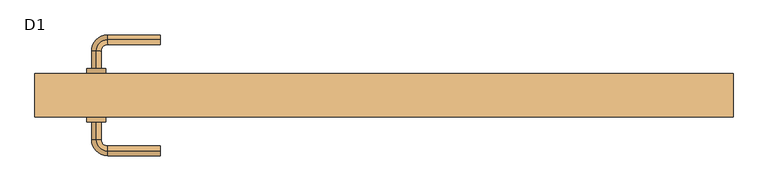
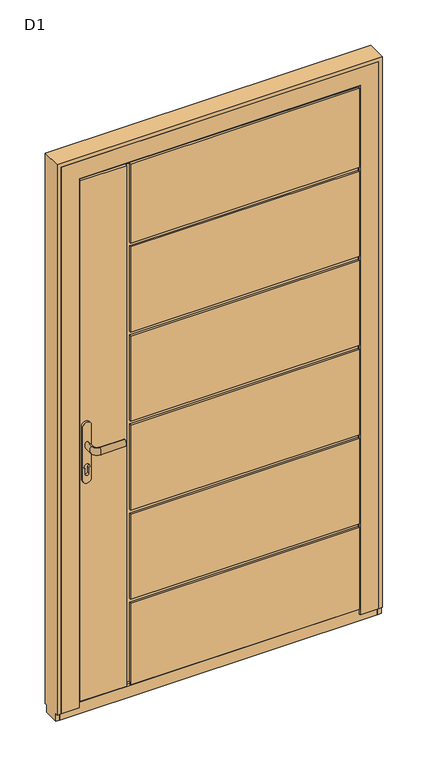
"""IFC4 building model written with IfcOpenShell, lengths in millimetres: door geometry, D1."""

from ifc_helpers import new_model, si_unit, point, frame, frame_2d, origin, place, context, project, spatial, polyline, circle_curve, ellipse_curve, trimmed, segment, composite_curve, outline, extrude, faceted_brep, source, transform, mapped, element, save
from ifc_brep_helpers import plane_surface, revolved_surface, extruded_surface, advanced_brep


def d1_d47119a4(model_context):
    return source(origin(), model_context, "Body", "SolidModel", [
        advanced_brep(
        [(-508.7, 104.0, 1064.0), (-508.7, 104.0, 1036.0), (-395.2, 155.0, 1064.0), (-395.2, 155.0, 1036.0), (-508.7, 135.0, 1036.0), (-508.7, 135.0, 1064.0), (-488.7, 155.0, 1036.0), (-488.7, 155.0, 1064.0)],
        [
            (0, 1, ellipse_curve(frame((-508.7, 104.0, 1050.0), z_axis=(0.0, -1.0, 0.0), x_axis=(0.0, 0.0, -1.0)), 14.0, 8.5)),
            (1, 0, ellipse_curve(frame((-508.7, 104.0, 1050.0), z_axis=(0.0, -1.0, 0.0), x_axis=(0.0, 0.0, -1.0)), 14.0, 8.5)),
            (2, 3, ellipse_curve(frame((-395.2, 155.0, 1050.0), z_axis=(1.0, 0.0, 0.0), x_axis=(0.0, 0.0, -1.0)), 14.0, 8.5)),
            (3, 2, ellipse_curve(frame((-395.2, 155.0, 1050.0), z_axis=(1.0, 0.0, 0.0), x_axis=(0.0, 0.0, -1.0)), 14.0, 8.5)),
            (1, 4),
            (4, 5, ellipse_curve(frame((-508.7, 135.0, 1050.0), z_axis=(0.0, -1.0, 0.0), x_axis=(0.0, 0.0, -1.0)), 14.0, 8.5)),
            (5, 0),
            (5, 4, ellipse_curve(frame((-508.7, 135.0, 1050.0), z_axis=(0.0, -1.0, 0.0), x_axis=(0.0, 0.0, -1.0)), 14.0, 8.5)),
            (6, 3),
            (2, 7),
            (7, 6, ellipse_curve(frame((-488.7, 155.0, 1050.0), z_axis=(1.0, 0.0, 0.0), x_axis=(0.0, 0.0, -1.0)), 14.0, 8.5)),
            (6, 7, ellipse_curve(frame((-488.7, 155.0, 1050.0), z_axis=(1.0, 0.0, 0.0), x_axis=(0.0, 0.0, -1.0)), 14.0, 8.5)),
            (7, 5, circle_curve(frame((-488.7, 135.0, 1064.0), z_axis=(0.0, 0.0, 1.0), x_axis=(-1.0, 0.0, 0.0)), 20.0)),
            (4, 6, circle_curve(frame((-488.7, 135.0, 1036.0), z_axis=(0.0, 0.0, -1.0), x_axis=(-1.0, 0.0, 0.0)), 20.0)),
        ],
        [
            plane_surface(frame((-508.7, 104.0, 1050.0), z_axis=(0.0, -1.0, 0.0), x_axis=(0.0, 0.0, 1.0))),
            plane_surface(frame((-395.2, 155.0, 1050.0), z_axis=(1.0, 0.0, 0.0), x_axis=(0.0, 0.0, 1.0))),
            extruded_surface(trimmed(ellipse_curve(frame((-508.7, 104.0, 1050.0), z_axis=(0.0, 1.0, 0.0), x_axis=(0.0, 0.0, -1.0)), 14.0, 8.5), [point((-508.7, 104.0, 1064.0))], [point((-508.7, 104.0, 1036.0))], True, "CARTESIAN"), (0.0, 31.0, 0.0), 31.0),
            extruded_surface(trimmed(ellipse_curve(frame((-508.7, 104.0, 1050.0), z_axis=(0.0, 1.0, 0.0), x_axis=(0.0, 0.0, -1.0)), 14.0, 8.5), [point((-508.7, 104.0, 1036.0))], [point((-508.7, 104.0, 1064.0))], True, "CARTESIAN"), (0.0, 31.0, 0.0), 31.0),
            extruded_surface(trimmed(ellipse_curve(frame((-488.7, 155.0, 1050.0), z_axis=(1.0, 0.0, 0.0), x_axis=(0.0, 0.0, -1.0)), 14.0, 8.5), [point((-488.7, 155.0, 1064.0))], [point((-488.7, 155.0, 1036.0))], True, "CARTESIAN"), (93.5, 0.0, 0.0), 93.5),
            extruded_surface(trimmed(ellipse_curve(frame((-488.7, 155.0, 1050.0), z_axis=(1.0, 0.0, 0.0), x_axis=(0.0, 0.0, -1.0)), 14.0, 8.5), [point((-488.7, 155.0, 1036.0))], [point((-488.7, 155.0, 1064.0))], True, "CARTESIAN"), (93.5, 0.0, 0.0), 93.5),
            revolved_surface(trimmed(ellipse_curve(frame((-508.7, 135.0, 1050.0), z_axis=(0.0, 1.0, 0.0), x_axis=(0.0, 0.0, -1.0)), 14.0, 8.5), [point((-508.7, 135.0, 1064.0))], [point((-508.7, 135.0, 1036.0))], True, "CARTESIAN"), (-488.7, 135.0, 1050.0), (0.0, 0.0, 1.0)),
            revolved_surface(trimmed(ellipse_curve(frame((-508.7, 135.0, 1050.0), z_axis=(0.0, 1.0, 0.0), x_axis=(0.0, 0.0, -1.0)), 14.0, 8.5), [point((-508.7, 135.0, 1036.0))], [point((-508.7, 135.0, 1064.0))], True, "CARTESIAN"), (-488.7, 135.0, 1050.0), (0.0, 0.0, 1.0)),
        ],
        [
            (0, [[1, 2]]),
            (1, [[3, 4]]),
            (2, [[5, 6, 7, -2]]),
            (3, [[-7, 8, -5, -1]]),
            (4, [[9, -3, 10, 11]]),
            (5, [[-10, -4, -9, 12]]),
            (6, [[-11, 13, -6, 14]]),
            (7, [[-12, -14, -8, -13]]),
        ],
    ),
        extrude(outline(composite_curve([segment(polyline([(1124.5, -525.2), (914.5, -525.2)]), True, "CONTINUOUS"), segment(trimmed(circle_curve(frame_2d((914.5, -508.7)), 16.5), [point((914.5, -525.2))], [point((914.5, -492.2))], False, "CARTESIAN"), True, "CONTINUOUS"), segment(polyline([(914.5, -492.2), (1124.5, -492.2)]), True, "CONTINUOUS"), segment(trimmed(circle_curve(frame_2d((1124.5, -508.7)), 16.5), [point((1124.5, -492.2))], [point((1124.5, -525.2))], False, "CARTESIAN"), True, "CONTINUOUS")], self_intersect=False), holes=[composite_curve([segment(trimmed(circle_curve(frame_2d((963.5537881, -508.7)), 10.0), [point((956.4123597, -515.7))], [point((956.4123597, -501.7))], True, "CARTESIAN"), True, "CONTINUOUS"), segment(polyline([(956.4123597, -501.7), (935.5537881, -501.7)]), True, "CONTINUOUS"), segment(trimmed(circle_curve(frame_2d((935.5537881, -508.7)), 7.0), [point((935.5537881, -501.7))], [point((935.5537881, -515.7))], True, "CARTESIAN"), True, "CONTINUOUS"), segment(polyline([(935.5537881, -515.7), (956.4123597, -515.7)]), True, "CONTINUOUS")], self_intersect=False)]), frame((0.0, 95.0, 0.0), z_axis=(0.0, 1.0, 0.0), x_axis=(0.0, 0.0, 1.0)), (0.0, 0.0, 1.0), 9.0),
        advanced_brep(
        [(-508.7, 9.0, 1064.0), (-508.7, 9.0, 1036.0), (-395.2, -42.0, 1064.0), (-395.2, -42.0, 1036.0), (-508.7, -22.0, 1064.0), (-508.7, -22.0, 1036.0), (-488.7, -42.0, 1036.0), (-488.7, -42.0, 1064.0)],
        [
            (0, 1, ellipse_curve(frame((-508.7, 9.0, 1050.0), z_axis=(0.0, 1.0, 0.0), x_axis=(0.0, 0.0, -1.0)), 14.0, 8.5)),
            (1, 0, ellipse_curve(frame((-508.7, 9.0, 1050.0), z_axis=(0.0, 1.0, 0.0), x_axis=(0.0, 0.0, -1.0)), 14.0, 8.5)),
            (2, 3, ellipse_curve(frame((-395.2, -42.0, 1050.0), z_axis=(1.0, 0.0, 0.0), x_axis=(0.0, 0.0, -1.0)), 14.0, 8.5)),
            (3, 2, ellipse_curve(frame((-395.2, -42.0, 1050.0), z_axis=(1.0, 0.0, 0.0), x_axis=(0.0, 0.0, -1.0)), 14.0, 8.5)),
            (0, 4),
            (4, 5, ellipse_curve(frame((-508.7, -22.0, 1050.0), z_axis=(0.0, 1.0, 0.0), x_axis=(0.0, 0.0, -1.0)), 14.0, 8.5)),
            (5, 1),
            (5, 4, ellipse_curve(frame((-508.7, -22.0, 1050.0), z_axis=(0.0, 1.0, 0.0), x_axis=(0.0, 0.0, -1.0)), 14.0, 8.5)),
            (6, 7, ellipse_curve(frame((-488.7, -42.0, 1050.0), z_axis=(1.0, 0.0, 0.0), x_axis=(0.0, 0.0, -1.0)), 14.0, 8.5)),
            (7, 2),
            (3, 6),
            (7, 6, ellipse_curve(frame((-488.7, -42.0, 1050.0), z_axis=(1.0, 0.0, 0.0), x_axis=(0.0, 0.0, -1.0)), 14.0, 8.5)),
            (6, 5, circle_curve(frame((-488.7, -22.0, 1036.0), z_axis=(0.0, 0.0, -1.0), x_axis=(-1.0, 0.0, 0.0)), 20.0)),
            (4, 7, circle_curve(frame((-488.7, -22.0, 1064.0), z_axis=(0.0, 0.0, 1.0), x_axis=(-1.0, 0.0, 0.0)), 20.0)),
        ],
        [
            plane_surface(frame((-508.7, 9.0, 1050.0), z_axis=(0.0, 1.0, 0.0), x_axis=(0.0, 0.0, 1.0))),
            plane_surface(frame((-395.2, -42.0, 1050.0), z_axis=(1.0, 0.0, 0.0), x_axis=(0.0, 0.0, 1.0))),
            extruded_surface(trimmed(ellipse_curve(frame((-508.7, -22.0, 1050.0), z_axis=(0.0, 1.0, 0.0), x_axis=(0.0, 0.0, -1.0)), 14.0, 8.5), [point((-508.7, -22.0, 1064.0))], [point((-508.7, -22.0, 1036.0))], True, "CARTESIAN"), (0.0, 31.0, 0.0), 31.0),
            extruded_surface(trimmed(ellipse_curve(frame((-508.7, -22.0, 1050.0), z_axis=(0.0, 1.0, 0.0), x_axis=(0.0, 0.0, -1.0)), 14.0, 8.5), [point((-508.7, -22.0, 1036.0))], [point((-508.7, -22.0, 1064.0))], True, "CARTESIAN"), (0.0, 31.0, 0.0), 31.0),
            extruded_surface(trimmed(ellipse_curve(frame((-395.2, -42.0, 1050.0), z_axis=(-1.0, 0.0, 0.0), x_axis=(0.0, 0.0, -1.0)), 14.0, 8.5), [point((-395.2, -42.0, 1064.0))], [point((-395.2, -42.0, 1036.0))], True, "CARTESIAN"), (-93.5, 0.0, 0.0), 93.5),
            extruded_surface(trimmed(ellipse_curve(frame((-395.2, -42.0, 1050.0), z_axis=(-1.0, 0.0, 0.0), x_axis=(0.0, 0.0, -1.0)), 14.0, 8.5), [point((-395.2, -42.0, 1036.0))], [point((-395.2, -42.0, 1064.0))], True, "CARTESIAN"), (-93.5, 0.0, 0.0), 93.5),
            revolved_surface(trimmed(ellipse_curve(frame((-508.7, -22.0, 1050.0), z_axis=(0.0, 1.0, 0.0), x_axis=(0.0, 0.0, -1.0)), 14.0, 8.5), [point((-508.7, -22.0, 1064.0))], [point((-508.7, -22.0, 1036.0))], True, "CARTESIAN"), (-488.7, -22.0, 1050.0), (0.0, 0.0, 1.0)),
            revolved_surface(trimmed(ellipse_curve(frame((-508.7, -22.0, 1050.0), z_axis=(0.0, 1.0, 0.0), x_axis=(0.0, 0.0, -1.0)), 14.0, 8.5), [point((-508.7, -22.0, 1036.0))], [point((-508.7, -22.0, 1064.0))], True, "CARTESIAN"), (-488.7, -22.0, 1050.0), (0.0, 0.0, 1.0)),
        ],
        [
            (0, [[1, 2]]),
            (1, [[3, 4]]),
            (2, [[-1, 5, 6, 7]]),
            (3, [[-2, -7, 8, -5]]),
            (4, [[9, 10, -4, 11]]),
            (5, [[12, -11, -3, -10]]),
            (6, [[13, -6, 14, -9]]),
            (7, [[-14, -8, -13, -12]]),
        ],
    ),
        extrude(outline(composite_curve([segment(polyline([(1124.5, -525.2), (914.5, -525.2)]), True, "CONTINUOUS"), segment(trimmed(circle_curve(frame_2d((914.5, -508.7)), 16.5), [point((914.5, -525.2))], [point((914.5, -492.2))], False, "CARTESIAN"), True, "CONTINUOUS"), segment(polyline([(914.5, -492.2), (1124.5, -492.2)]), True, "CONTINUOUS"), segment(trimmed(circle_curve(frame_2d((1124.5, -508.7)), 16.5), [point((1124.5, -492.2))], [point((1124.5, -525.2))], False, "CARTESIAN"), True, "CONTINUOUS")], self_intersect=False), holes=[composite_curve([segment(trimmed(circle_curve(frame_2d((963.5537881, -508.7)), 10.0), [point((956.4123597, -515.7))], [point((956.4123597, -501.7))], True, "CARTESIAN"), True, "CONTINUOUS"), segment(polyline([(956.4123597, -501.7), (935.5537881, -501.7)]), True, "CONTINUOUS"), segment(trimmed(circle_curve(frame_2d((935.5537881, -508.7)), 7.0), [point((935.5537881, -501.7))], [point((935.5537881, -515.7))], True, "CARTESIAN"), True, "CONTINUOUS"), segment(polyline([(935.5537881, -515.7), (956.4123597, -515.7)]), True, "CONTINUOUS")], self_intersect=False)]), frame((0.0, 9.0, 0.0), z_axis=(0.0, 1.0, 0.0), x_axis=(0.0, 0.0, 1.0)), (0.0, 0.0, 1.0), 9.0),
        faceted_brep([(-338.7, 25.0, 366.5833337), (-338.7, 25.0, 708.166667), (528.7, 25.0, 708.166667), (528.7, 25.0, 723.166667), (-338.7, 25.0, 723.166667), (-338.7, 25.0, 1064.7500004), (528.7, 25.0, 1064.7500004), (528.7, 25.0, 1079.7500004), (-338.7, 25.0, 1079.7500004), (-338.7, 25.0, 1421.3333337), (528.7, 25.0, 1421.3333337), (528.7, 25.0, 1436.3333337), (-338.7, 25.0, 1436.3333337), (-338.7, 25.0, 1777.916667), (528.7, 25.0, 1777.916667), (528.7, 25.0, 1792.916667), (-338.7, 25.0, 1792.916667), (-338.7, 25.0, 2109.5000003), (-353.7, 25.0, 2109.5000003), (-353.7, 25.0, 35.0), (-338.7, 25.0, 35.0), (-338.7, 25.0, 351.5833337), (528.7, 25.0, 351.5833337), (528.7, 25.0, 366.5833337), (-338.7, 18.0, 366.5833337), (-338.7, 18.0, 708.166667), (528.7, 18.0, 708.166667), (528.7, 27.0002302, 2109.5000003), (528.7, 18.0, 2109.5000003), (528.7, 18.0, 1792.916667), (528.7, 18.0, 1777.916667), (528.7, 18.0, 1436.3333337), (528.7, 18.0, 1421.3333337), (528.7, 18.0, 1079.7500004), (528.7, 18.0, 1064.7500004), (528.7, 18.0, 723.166667), (528.7, 18.0, 366.5833337), (528.7, 18.0, 351.5833337), (528.7, 18.0, 24.0), (528.7, 19.9979528, 24.0), (528.7, 19.9979528, 35.0), (528.7, 27.0002302, 35.0), (-338.7, 18.0, 723.166667), (-338.7, 18.0, 1064.7500004), (-338.7, 18.0, 1079.7500004), (-338.7, 18.0, 1421.3333337), (-353.7, 18.0, 2109.5000003), (-353.7, 18.0, 24.0), (-353.7, 19.9979528, 24.0), (-353.7, 19.9979528, 35.0), (-338.7, 19.9979528, 35.0), (-528.7, 19.9979528, 35.0), (-528.7, 27.0002302, 35.0), (-338.7, 18.0, 351.5833337), (-338.7, 19.9979528, 24.0), (-338.7, 18.0, 24.0), (-528.7, 19.9979528, 24.0), (-528.7, 18.0, 24.0), (-528.7, 18.0, 2109.5000003), (-338.7, 18.0, 1777.916667), (-338.7, 18.0, 1436.3333337), (-338.7, 18.0, 2109.5000003), (-338.7, 18.0, 1792.916667), (553.7, 95.0, 10.0000003), (553.7, 92.0, 10.0000003), (-338.7, 92.0, 10.0000003), (-338.7, 95.0, 10.0000003), (-553.7, 92.0, 10.0000003), (-553.7, 95.0, 10.0000003), (-353.7, 95.0, 10.0000003), (-353.7, 92.0, 10.0000003), (553.7, 95.0, 351.5833337), (553.7, 92.0, 351.5833337), (553.7, 95.0, 366.5833337), (553.7, 95.0, 708.166667), (553.7, 92.0, 708.166667), (553.7, 92.0, 366.5833337), (553.7, 95.0, 1079.7500004), (553.7, 95.0, 1421.3333337), (553.7, 92.0, 1421.3333337), (553.7, 92.0, 1079.7500004), (553.7, 95.0, 723.166667), (553.7, 95.0, 1064.7500004), (553.7, 92.0, 1064.7500004), (553.7, 92.0, 723.166667), (553.7, 95.0, 1436.3333337), (553.7, 95.0, 1777.916667), (553.7, 92.0, 1777.916667), (553.7, 92.0, 1436.3333337), (553.7, 95.0, 2134.5000003), (553.7, 92.0, 2134.5000003), (553.7, 92.0, 1792.916667), (553.7, 95.0, 1792.916667), (538.2, 92.0, 351.5833337), (538.2, 92.0, 25.5), (-338.7, 92.0, 25.5), (538.2, 92.0, 708.166667), (538.2, 92.0, 366.5833337), (538.2, 92.0, 1421.3333337), (538.2, 92.0, 1079.7500004), (538.2, 92.0, 1064.7500004), (538.2, 92.0, 723.166667), (538.2, 92.0, 1777.916667), (538.2, 92.0, 1436.3333337), (-338.7, 92.0, 2134.5000003), (-338.7, 92.0, 2119.0000003), (538.2, 92.0, 2119.0000003), (538.2, 92.0, 1792.916667), (-538.2, 92.0, 25.5), (-538.2, 92.0, 2119.0000003), (-353.7, 92.0, 2119.0000003), (-353.7, 92.0, 2134.5000003), (-553.7, 92.0, 2134.5000003), (-353.7, 92.0, 25.5), (-338.7, 88.0, 351.5833337), (-338.7, 95.0, 351.5833337), (-338.7, 88.0, 25.5), (-338.7, 95.0, 366.5833337), (-338.7, 95.0, 708.166667), (-338.7, 95.0, 1079.7500004), (-338.7, 95.0, 1421.3333337), (-338.7, 95.0, 723.166667), (-338.7, 95.0, 1064.7500004), (-338.7, 95.0, 1436.3333337), (-338.7, 95.0, 1777.916667), (-338.7, 95.0, 1792.916667), (-338.7, 95.0, 2134.5000003), (-553.7, 95.0, 2134.5000003), (-353.7, 95.0, 2134.5000003), (-353.7, 88.0, 2119.0000003), (-353.7, 88.0, 25.5), (-528.7, 27.0002302, 2109.5000003), (538.2, 27.0002302, 2119.0000003), (-538.2, 27.0002302, 2119.0000003), (-538.2, 27.0002302, 25.5), (538.2, 27.0002302, 25.5), (538.2, 88.0, 351.5833337), (538.2, 88.0, 366.5833337), (538.2, 88.0, 708.166667), (538.2, 88.0, 723.166667), (538.2, 88.0, 1064.7500004), (538.2, 88.0, 1079.7500004), (538.2, 88.0, 1421.3333337), (538.2, 88.0, 1436.3333337), (538.2, 88.0, 1777.916667), (538.2, 88.0, 1792.916667), (-338.7, 88.0, 1777.916667), (-338.7, 88.0, 1436.3333337), (-338.7, 88.0, 1421.3333337), (-338.7, 88.0, 1079.7500004), (-338.7, 88.0, 1064.7500004), (-338.7, 88.0, 723.166667), (-338.7, 88.0, 708.166667), (-338.7, 88.0, 366.5833337), (-338.7, 88.0, 2119.0000003), (-338.7, 88.0, 1792.916667)], [[[0, 1, 2, 3, 4, 5, 6, 7, 8, 9, 10, 11, 12, 13, 14, 15, 16, 17, 18, 19, 20, 21, 22, 23]], [[1, 0, 24, 25]], [[1, 25, 26, 2]], [[27, 28, 29, 15, 14, 30, 31, 11, 10, 32, 33, 7, 6, 34, 35, 3, 2, 26, 36, 23, 22, 37, 38, 39, 40, 41]], [[42, 4, 3, 35]], [[5, 4, 42, 43]], [[5, 43, 34, 6]], [[44, 8, 7, 33]], [[9, 8, 44, 45]], [[19, 18, 46, 47, 48, 49]], [[41, 40, 50, 20, 19, 49, 51, 52]], [[53, 21, 20, 50, 54, 55]], [[21, 53, 37, 22]], [[24, 0, 23, 36]], [[40, 39, 54, 50]], [[56, 51, 49, 48]], [[39, 38, 55, 54]], [[57, 56, 48, 47]], [[33, 32, 45, 44]], [[35, 34, 43, 42]], [[36, 26, 25, 24]], [[55, 38, 37, 53]], [[58, 57, 47, 46]], [[31, 30, 59, 60]], [[28, 61, 62, 29]], [[63, 64, 65, 66]], [[67, 68, 69, 70]], [[64, 63, 71, 72]], [[73, 74, 75, 76]], [[77, 78, 79, 80]], [[81, 82, 83, 84]], [[85, 86, 87, 88]], [[89, 90, 91, 92]], [[65, 64, 72, 93, 94, 95]], [[76, 75, 96, 97]], [[80, 79, 98, 99]], [[84, 83, 100, 101]], [[88, 87, 102, 103]], [[90, 104, 105, 106, 107, 91]], [[108, 109, 110, 111, 112, 67, 70, 113]], [[114, 115, 66, 65, 95, 116]], [[63, 66, 115, 71]], [[74, 73, 117, 118]], [[78, 77, 119, 120]], [[82, 81, 121, 122]], [[86, 85, 123, 124]], [[89, 92, 125, 126]], [[68, 127, 128, 69]], [[68, 67, 112, 127]], [[129, 130, 113, 70, 69, 128, 111, 110]], [[58, 131, 52, 51, 56, 57]], [[132, 133, 134, 135], [131, 27, 41, 52]], [[106, 132, 135, 94, 93, 136, 137, 97, 96, 138, 139, 101, 100, 140, 141, 99, 98, 142, 143, 103, 102, 144, 145, 107]], [[94, 135, 134, 108, 113, 130, 116, 95]], [[133, 109, 108, 134]], [[146, 147, 143, 142, 148, 149, 141, 140, 150, 151, 139, 138, 152, 153, 137, 136, 114, 116, 130, 129, 154, 155, 145, 144]], [[149, 148, 120, 119]], [[149, 119, 77, 80, 99, 141]], [[122, 150, 140, 100, 83, 82]], [[151, 150, 122, 121]], [[151, 121, 81, 84, 101, 139]], [[118, 152, 138, 96, 75, 74]], [[153, 152, 118, 117]], [[153, 117, 73, 76, 97, 137]], [[115, 114, 136, 93, 72, 71]], [[9, 45, 32, 10]], [[60, 12, 11, 31]], [[13, 12, 60, 59]], [[13, 59, 30, 14]], [[62, 16, 15, 29]], [[16, 62, 61, 17]], [[124, 146, 144, 102, 87, 86]], [[125, 155, 154, 105, 104, 126]], [[120, 148, 142, 98, 79, 78]], [[147, 123, 85, 88, 103, 143]], [[147, 146, 124, 123]], [[155, 125, 92, 91, 107, 145]], [[90, 89, 126, 104]], [[127, 112, 111, 128]], [[132, 106, 105, 154, 129, 110, 109, 133]], [[27, 131, 58, 46, 18, 17, 61, 28]]]),
        faceted_brep([(-602.25, 95.0, 0.0), (-557.75, 95.0, 0.0), (-557.75, 86.0, 0.0), (-602.25, 85.9997571, 0.0), (-548.25, 22.5000042, 0.0), (-532.75, 22.5000042, 0.0), (-532.75, 18.0, 0.0), (-602.25, 18.0, 0.0), (-602.25, 27.0, 0.0), (-548.25, 27.0, 0.0), (602.25, 18.0, 0.0), (532.75, 18.0, 0.0), (532.75, 22.5000042, 0.0), (548.25, 22.5000042, 0.0), (548.25, 27.0, 0.0), (602.25, 27.0, 0.0), (557.75, 86.0, 0.0), (557.75, 95.0, 0.0), (602.25, 95.0, 0.0), (602.25, 85.9997571, 0.0), (-602.25, 18.0, 2189.5), (-602.25, 95.0, 2189.5), (-602.25, 85.9997571, -30.0), (-602.25, 27.0, -30.0), (602.25, 95.0, 2189.5), (557.75, 95.0, 2145.0), (-557.75, 95.0, 2145.0), (602.25, 18.0, 2189.5), (602.25, 27.0, -30.0), (602.25, 85.9997571, -30.0), (-532.75, 18.0, 2120.0), (532.75, 18.0, 2120.0), (-548.25, 86.0, 2135.5), (-548.25, 22.5000042, 2135.5), (-548.25, 27.0, 14.5), (-548.25, 86.0, 14.5), (548.25, 86.0, 2135.5), (548.25, 22.5000042, 2135.5), (548.25, 86.0, 14.5), (548.25, 27.0, 14.5), (-557.75, 86.0, 2145.0), (557.75, 86.0, 2145.0), (532.75, 22.5000042, 2120.0), (-532.75, 22.5000042, 2120.0)], [[[0, 1, 2, 3]], [[4, 5, 6, 7, 8, 9]], [[10, 11, 12, 13, 14, 15]], [[16, 17, 18, 19]], [[7, 20, 21, 0, 3, 22, 23, 8]], [[1, 0, 21, 24, 18, 17, 25, 26]], [[21, 20, 27, 24]], [[18, 24, 27, 10, 15, 28, 29, 19]], [[7, 6, 30, 31, 11, 10, 27, 20]], [[32, 33, 4, 9, 34, 35]], [[33, 32, 36, 37]], [[37, 36, 38, 39, 14, 13]], [[40, 2, 1, 26]], [[16, 19, 29, 22, 3, 2, 40, 41], [36, 32, 35, 38]], [[5, 4, 33, 37, 13, 12, 42, 43]], [[6, 5, 43, 30]], [[26, 25, 41, 40]], [[31, 30, 43, 42]], [[17, 16, 41, 25]], [[12, 11, 31, 42]], [[23, 28, 15, 14, 39, 34, 9, 8]], [[38, 35, 34, 39]], [[23, 22, 29, 28]]]),
        faceted_brep([(-602.25, 86.0, -30.0), (-602.25, 27.0, -30.0), (-617.25, 27.0, -30.0), (-617.25, 86.0, -30.0), (-602.25, 95.0, 2189.5), (-602.25, 18.0, 2189.5), (-602.25, 18.0, 0.0), (-602.25, 27.0, 0.0), (-602.25, 86.0, 0.0), (-602.25, 95.0, 0.0), (617.25, 27.0, 0.0), (602.25, 27.0, 0.0), (602.25, 27.0, -30.0), (617.25, 27.0, -30.0), (-617.25, 27.0, 0.0), (-617.25, 18.0, 2204.5), (-617.25, 95.0, 2204.5), (-617.25, 95.0, 0.0), (-617.25, 86.0, 0.0), (-617.25, 18.0, 0.0), (602.25, 86.0, 0.0), (617.25, 86.0, 0.0), (617.25, 86.0, -30.0), (602.25, 86.0, -30.0), (602.25, 18.0, 2189.5), (602.25, 95.0, 2189.5), (602.25, 95.0, 0.0), (602.25, 18.0, 0.0), (617.25, 95.0, 2204.5), (617.25, 95.0, 0.0), (617.25, 18.0, 0.0), (617.25, 18.0, 2204.5)], [[[0, 1, 2, 3]], [[4, 5, 6, 7, 1, 0, 8, 9]], [[10, 11, 12, 13]], [[7, 14, 2, 1]], [[15, 16, 17, 18, 3, 2, 14, 19]], [[20, 21, 22, 23]], [[18, 8, 0, 3]], [[24, 25, 26, 20, 23, 12, 11, 27]], [[25, 4, 9, 17, 16, 28, 29, 26]], [[21, 20, 26, 29]], [[8, 18, 17, 9]], [[22, 13, 12, 23]], [[11, 10, 30, 27]], [[14, 7, 6, 19]], [[5, 24, 27, 30, 31, 15, 19, 6]], [[28, 31, 30, 10, 13, 22, 21, 29]], [[5, 4, 25, 24]], [[16, 15, 31, 28]]]),
    ])


if __name__ == "__main__":
    model = new_model("IFC4")
    model_context = context("Model", 3, world=origin())
    ifc_project = project(units=[si_unit("LENGTHUNIT", "METRE", prefix="MILLI")], contexts=[model_context])
    site = spatial("IfcSite", under=ifc_project)
    building = spatial("IfcBuilding", under=site)
    placement = place(None, origin())
    d1_shape = d1_d47119a4(model_context)
    element("IfcDoor", 1, ObjectType="D1", at=placement, inside=building, context=model_context, shape_type="MappedRepresentation", body=[
        mapped(d1_shape, transform((0.0, 0.0, 0.0), x_axis=(1.0, 0.0, 0.0), y_axis=(0.0, 1.0, 0.0), z_axis=(0.0, 0.0, 1.0))),
    ])
    save(model, "model.ifc")

# Revit data of these elements
# Type "D1"
#   Type Mark = "22"
#   Water resistance = "up to Class E900, EN 12208:2001"
#   Uniclass2015Version = "v1.21"
#   Uniclass2015Reference = "Ss_25_30_20_30"
#   Uniclass2015Description = "Frame and door leaf system"
#   URL = "www.aluprof.eu"
#   Type IFC Predefined Type = "USERDEFINED"
#   Right-hand / Left-hand door [instance default] = ""
#   Resistance to wind load = "up to Class C5/B5, EN 12210:2001"
#   Insert type = "ST"
#   Hardware [instance default] = ""
#   Product page = "https://aluprof.eu/en/architects/offer/window-and-door-systems/panel-doors#visualisation"
#   Operation = "SinglePanelOutwardOpening"
#   Opening type = "Outward"
#   NBSReference = "25-50-20/125"
#   NBSDescription = "Frame and door leaf system"
#   Important = "The actual acceptable construction dimensions are dependent on the selection of profiles and hardware, glazing type, construction weight and the construction’s operating conditions. These should be determined by a suitably qualified person, and using ALUPROF’s calculation software"
#   IfcExportType = "USERDEFINED"
#   IfcExportAs = "IfcDoorType"
#   Handle type [instance default] = ""
#   Manufacturer = "ALUPROF"
#   Export Type to IFC As = "IfcDoorType"
#   Door sill type [instance default] = ""
#   Description = "External single-leaf panel door outward opening"
#   Model = "MB-86 ST Panel Door AD07"
#   Content of the recyclate in the material = "69.2"
#   COBie.Type.WarrantyDurationParts = ""
#   COBie.Type.Name = ""
#   COBie.Type.Manufacturer = "ALUPROF S.A."
#   COBie.Space.Name = ""
#   COBie.Floor.Name = ""
#   COBie.Facility.Name = ""
#   COBie.CreatedOn = ""
#   COBie.Component.WarrantyStartDate = ""
#   COBie.Component.Name = "MB-86 ST Panel Door AD07"
#   Burglar resistance = "RC2"
#   Air permeability = "up to Class 4, EN 12207:2001"
#   Width of the active leaf = 1107.4 mm
#   Placement in wall = 20 mm
#   Thickness = 77 mm
#   Height of the opening sash = 2124.5 mm
#   Handle Offset = 1050 mm
#   Glazing thickness = 48 mm
#   Rough Height = 2250.7 mm
#   Rough Width = 1234.5 mm
#   Height = 2189.5 mm
#   Width = 1204.5 mm
#   Construction depth = 77 mm
#   Clear opening width = 1000 mm
#   Clear opening height = 2100 mm
#   Height of the array = 341.583 mm
#   Schedule No. [instance default] = 1
#   Handrail = no
#   IsExternal = yes
#   Handle = yes
#   Door closer [instance default] = no
#   Function = 1
#   COBie.Type = yes
#   COBie = yes
#   Access control [instance default] = no
#   Panel = element 260956
#   Wall Closure = (empty or 0)
